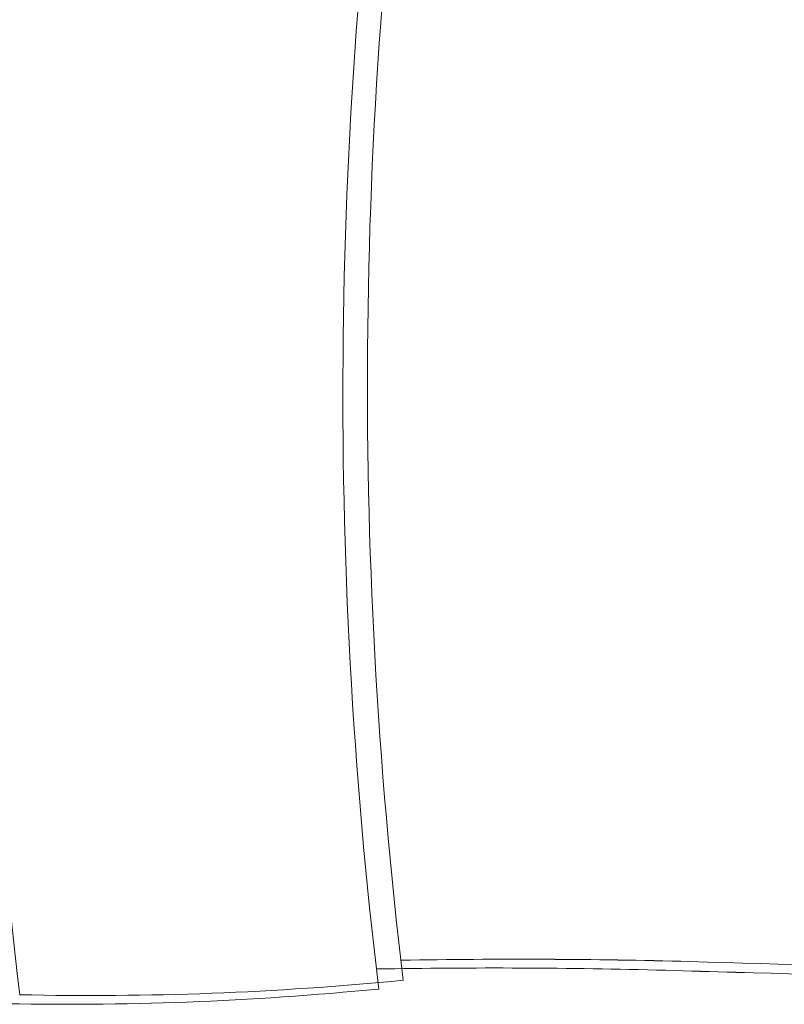
# Model space of a CAD drawing. Units: inches. Extents: x 1901 to 2863, y 888 to 2433.
# Tile 56 of 91: x 2051 to 2073, y 2132 to 2161. Entities that reach past the tile are written whole.
import ezdxf

# ---------------------------------------------------------------- set-up
doc = ezdxf.new("R2010")
doc.units = ezdxf.units.IN
doc.layers.add('A-FURN', color=8, linetype='Continuous', lineweight=18)

# ---------------------------------------------------------------- blocks, each defined once
blk = doc.blocks.new('BED-DOUBLE')
for centre, radius, start, end in [((176.248, 20.155), 144.857, 171.78449, 186.90062), ((176.248, 20.155), 144.857, 171.78449, 186.90062), ((175.53, 19.899), 144.857, 171.78449, 186.90062), ((175.53, 19.899), 144.857, 171.78449, 186.90062), ((205.143, 24.2), 185.219, 176.08655, 186.78213), ((35.744, -187.624), 190.991, 88.4762, 91.00819), ((35.744, -187.625), 190.991, 88.4762, 91.00819), ((57.571, 544.554), 541.514, 268.22771, 271.71854), ((57.571, 544.554), 541.514, 268.22771, 271.71854), ((35.026, -187.881), 190.991, 88.4762, 91.00819), ((35.026, -187.881), 190.991, 88.4762, 91.00819), ((56.853, 544.298), 541.514, 268.22771, 271.71854), ((56.853, 544.297), 541.514, 268.22771, 271.71854), ((23.307, 95.835), 93.531, 268.72178, 275.60397), ((23.307, 95.835), 93.531, 268.72178, 275.60397), ((22.589, 95.579), 93.531, 268.72178, 275.60397), ((22.589, 95.579), 93.531, 268.72178, 275.60397)]:
    blk.add_arc(centre, radius, start, end)

msp = doc.modelspace()

# ---------------------------------------------------------------- block references
at = {"layer": 'A-FURN'}
msp.add_blockref('BED-DOUBLE', (2029.4, 2130), dxfattribs=at)

doc.saveas('drawing.dxf')
